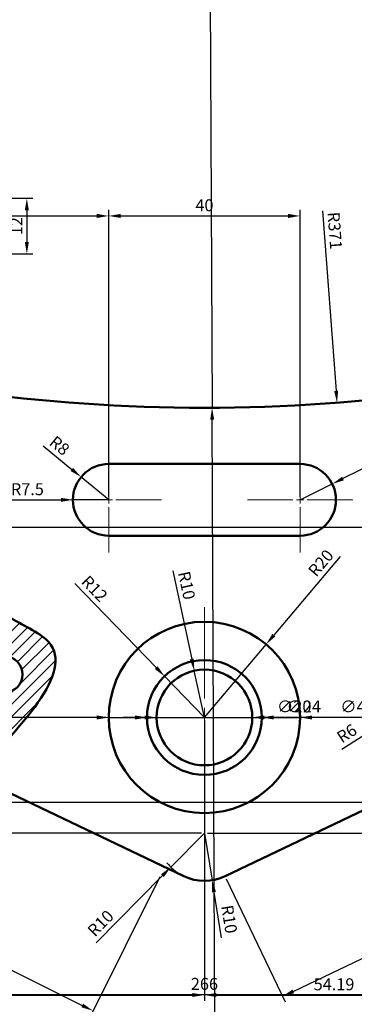
# Model space of a CAD drawing. Units: millimetres. Extents: x 1605 to 2079, y 1280 to 1879.
# Tile 4 of 7: x 1745 to 1815, y 1384 to 1589. Entities that reach past the tile are written whole.
import ezdxf

# ---------------------------------------------------------------- set-up
doc = ezdxf.new("R2010")
doc.units = ezdxf.units.MM
doc.linetypes.add('CENTER2', pattern=[28.575, 19.05, -3.175, 3.175, -3.175])
for name, color, linetype, lineweight in [('M-CNTR', 1, 'CENTER2', 18), ('M-DIMS', 2, 'Continuous', 25), ('M-HATC', 8, 'Continuous', 18), ('M-OUTL', 7, 'Continuous', 50)]:
    doc.layers.add(name, color=color, linetype=linetype, lineweight=lineweight)
doc.styles.get("Standard").update_dxf_attribs({"font": 'arial.ttf'})
doc.dimstyles.new('ISO-25', dxfattribs={"dimtxt": 2.5, "dimasz": 2.5, "dimexe": 1.25, "dimexo": 0.625, "dimtad": 1, "dimdec": 0, "dimtxsty": 'Standard', "dimcen": 2.5, "dimadec": 0, "dimazin": 0, "dimtfac": 1, "dimtdec": 0, "dimtmove": 0, "dimatfit": 3, "dimfxl": 1, "dimarcsym": 0})

# ---------------------------------------------------------------- blocks, each defined once
blk = doc.blocks.new('*U1')
at = {"layer": 'M-CNTR', "color": 0, "transparency": 16777216}
for p, q in [((0, 4), (0, 23.5)), ((-23.5, 0), (-4, 0)), ((4, 0), (23.5, 0)), ((0, -23.5), (0, -4))]:
    blk.add_line(p, q, dxfattribs=at)
at = {"layer": 'M-CNTR', "color": 0, "linetype": 'Continuous', "transparency": 16777216}
for p, q in [((-2, 0), (2, 0)), ((0, -2), (0, 2))]:
    blk.add_line(p, q, dxfattribs=at)
blk = doc.blocks.new('*U4')
at = {"layer": 'M-CNTR', "color": 0, "transparency": 16777216}
for p, q in [((0, 1.5), (0, 11)), ((-11, 0), (-1.5, 0)), ((1.5, 0), (11, 0)), ((0, -11), (0, -1.5))]:
    blk.add_line(p, q, dxfattribs=at)
at = {"layer": 'M-CNTR', "color": 0, "linetype": 'Continuous', "transparency": 16777216}
for p, q in [((-0.75, 0), (0.75, 0)), ((0, -0.75), (0, 0.75))]:
    blk.add_line(p, q, dxfattribs=at)
blk = doc.blocks.new('*U5')
at = {"layer": 'M-CNTR', "color": 0, "transparency": 16777216}
for p, q in [((0, 1.5), (0, 11)), ((-11, 0), (-1.5, 0)), ((1.5, 0), (11, 0)), ((0, -11), (0, -1.5))]:
    blk.add_line(p, q, dxfattribs=at)
at = {"layer": 'M-CNTR', "color": 0, "linetype": 'Continuous', "transparency": 16777216}
for p, q in [((-0.75, 0), (0.75, 0)), ((0, -0.75), (0, 0.75))]:
    blk.add_line(p, q, dxfattribs=at)
blk = doc.blocks.new('*D8')
at = {"layer": 'Defpoints', "color": 0, "transparency": 16777216}
for p in [(1738.95, 1552.02), (1738.95, 1540.38), (1746.29, 1540.38)]:
    blk.add_point(p, dxfattribs=at)
at = {"layer": 'M-DIMS', "color": 0, "lineweight": -2, "transparency": 16777216}
for p, q in [((1739.57, 1552.02), (1747.54, 1552.02)), ((1746.29, 1549.52), (1746.29, 1542.88)), ((1739.57, 1540.38), (1747.54, 1540.38))]:
    blk.add_line(p, q, dxfattribs=at)
at = {"layer": 'M-DIMS', "color": 0, "transparency": 16777216}
for points in [[(1745.87, 1549.52), (1746.71, 1549.52), (1746.29, 1552.02)], [(1745.87, 1542.88), (1746.71, 1542.88), (1746.29, 1540.38)]]:
    blk.add_solid(points, dxfattribs=at)
at = {"layer": 'M-DIMS', "color": 0, "transparency": 16777216, "insert": (1744.41, 1546.2), "char_height": 2.5, "attachment_point": 5, "rotation": 90}
blk.add_mtext('12', dxfattribs=at)
blk = doc.blocks.new('*D12')
at = {"layer": 'Defpoints', "color": 0, "transparency": 16777216}
for p in [(1650.42, 1488.98), (1916.42, 1488.98), (1916.42, 1385.56)]:
    blk.add_point(p, dxfattribs=at)
at = {"layer": 'M-DIMS', "color": 0, "lineweight": -2, "transparency": 16777216}
for p, q in [((1650.42, 1488.36), (1650.42, 1384.31)), ((1916.42, 1488.36), (1916.42, 1384.31)), ((1652.92, 1385.56), (1913.92, 1385.56))]:
    blk.add_line(p, q, dxfattribs=at)
at = {"layer": 'M-DIMS', "color": 0, "transparency": 16777216}
for points in [[(1652.92, 1385.97), (1652.92, 1385.14), (1650.42, 1385.56)], [(1913.92, 1385.97), (1913.92, 1385.14), (1916.42, 1385.56)]]:
    blk.add_solid(points, dxfattribs=at)
at = {"layer": 'M-DIMS', "color": 0, "transparency": 16777216, "insert": (1783.42, 1387.46), "char_height": 2.5, "attachment_point": 5}
blk.add_mtext('266', dxfattribs=at)
blk = doc.blocks.new('*D13')
at = {"layer": 'Defpoints', "color": 0, "transparency": 16777216}
for p in [(1783.42, 1419.31), (1776.39, 1412.2)]:
    blk.add_point(p, dxfattribs=at)
at = {"layer": 'M-DIMS', "color": 0, "lineweight": -2, "transparency": 16777216}
for p, q in [((1783.42, 1419.31), (1776.39, 1412.2)), ((1760.75, 1396.34), (1774.64, 1410.42))]:
    blk.add_line(p, q, dxfattribs=at)
blk.add_arc((1783.42, 1419.31), 10, 218.2245, 240.8957, dxfattribs=at)
at = {"layer": 'M-DIMS', "color": 0, "transparency": 16777216}
blk.add_solid([(1774.34, 1410.71), (1774.93, 1410.12), (1776.39, 1412.2)], dxfattribs=at)
at = {"layer": 'M-DIMS', "color": 0, "transparency": 16777216, "insert": (1761.93, 1400.24), "char_height": 2.5, "attachment_point": 5, "rotation": 45.3865}
blk.add_mtext('R10', dxfattribs=at)
blk = doc.blocks.new('*D17')
at = {"layer": 'Defpoints', "color": 0, "transparency": 16777216}
for p in [(1783.42, 1878.81), (1811.14, 1509.27)]:
    blk.add_point(p, dxfattribs=at)
at = {"layer": 'M-DIMS', "color": 0, "lineweight": -2, "transparency": 16777216}
blk.add_line((1808.13, 1549.43), (1810.96, 1511.76), dxfattribs=at)
at = {"layer": 'M-DIMS', "color": 0, "transparency": 16777216}
blk.add_solid([(1811.37, 1511.8), (1810.54, 1511.73), (1811.14, 1509.27)], dxfattribs=at)
at = {"layer": 'M-DIMS', "color": 0, "transparency": 16777216, "insert": (1810.35, 1545.24), "char_height": 2.5, "attachment_point": 5, "rotation": 274.2909}
blk.add_mtext('R371', dxfattribs=at)
blk = doc.blocks.new('*D19')
at = {"layer": 'Defpoints', "color": 0, "transparency": 16777216}
for p in [(1796.31, 1458.77), (1783.42, 1443.48)]:
    blk.add_point(p, dxfattribs=at)
at = {"layer": 'M-DIMS', "color": 0, "lineweight": -2, "transparency": 16777216}
for p, q in [((1811.78, 1477.12), (1797.92, 1460.68)), ((1783.42, 1443.48), (1796.31, 1458.77))]:
    blk.add_line(p, q, dxfattribs=at)
at = {"layer": 'M-DIMS', "color": 0, "transparency": 16777216}
blk.add_solid([(1797.6, 1460.95), (1798.24, 1460.41), (1796.31, 1458.77)], dxfattribs=at)
at = {"layer": 'M-DIMS', "color": 0, "transparency": 16777216, "insert": (1808, 1475.58), "char_height": 2.5, "attachment_point": 5, "rotation": 49.8645}
blk.add_mtext('R20', dxfattribs=at)
blk = doc.blocks.new('*D20')
at = {"layer": 'Defpoints', "color": 0, "transparency": 16777216}
for p in [(1775.07, 1452.1), (1783.42, 1443.48)]:
    blk.add_point(p, dxfattribs=at)
at = {"layer": 'M-DIMS', "color": 0, "lineweight": -2, "transparency": 16777216}
for p, q in [((1756.34, 1471.47), (1773.33, 1453.9)), ((1783.42, 1443.48), (1775.07, 1452.1))]:
    blk.add_line(p, q, dxfattribs=at)
at = {"layer": 'M-DIMS', "color": 0, "transparency": 16777216}
blk.add_solid([(1773.63, 1454.19), (1773.03, 1453.61), (1775.07, 1452.1)], dxfattribs=at)
at = {"layer": 'M-DIMS', "color": 0, "transparency": 16777216, "insert": (1760.2, 1470.19), "char_height": 2.5, "attachment_point": 5, "rotation": 314.0509}
blk.add_mtext('R12', dxfattribs=at)
blk = doc.blocks.new('*D21')
at = {"layer": 'Defpoints', "color": 0, "transparency": 16777216}
for p in [(1781.3, 1453.25), (1783.42, 1443.48)]:
    blk.add_point(p, dxfattribs=at)
at = {"layer": 'M-DIMS', "color": 0, "lineweight": -2, "transparency": 16777216}
for p, q in [((1776.78, 1474.15), (1780.77, 1455.7)), ((1783.42, 1443.48), (1781.3, 1453.25))]:
    blk.add_line(p, q, dxfattribs=at)
at = {"layer": 'M-DIMS', "color": 0, "transparency": 16777216}
blk.add_solid([(1781.18, 1455.78), (1780.36, 1455.61), (1781.3, 1453.25)], dxfattribs=at)
at = {"layer": 'M-DIMS', "color": 0, "transparency": 16777216, "insert": (1779.4, 1471.02), "char_height": 2.5, "attachment_point": 5, "rotation": 282.212}
blk.add_mtext('R10', dxfattribs=at)
blk = doc.blocks.new('*D22')
at = {"layer": 'Defpoints', "color": 0, "transparency": 16777216}
for p in [(1810.14, 1492.31), (1803.42, 1488.98)]:
    blk.add_point(p, dxfattribs=at)
at = {"layer": 'M-DIMS', "color": 0, "lineweight": -2, "transparency": 16777216}
for p, q in [((1824.04, 1499.19), (1812.38, 1493.42)), ((1803.42, 1488.98), (1810.14, 1492.31))]:
    blk.add_line(p, q, dxfattribs=at)
at = {"layer": 'M-DIMS', "color": 0, "transparency": 16777216}
blk.add_solid([(1812.19, 1493.79), (1812.56, 1493.05), (1810.14, 1492.31)], dxfattribs=at)
at = {"layer": 'M-DIMS', "color": 0, "transparency": 16777216, "insert": (1820.82, 1499.72), "char_height": 2.5, "attachment_point": 5, "rotation": 26.3503}
blk.add_mtext('R8', dxfattribs=at)
blk = doc.blocks.new('*D23')
at = {"layer": 'Defpoints', "color": 0, "transparency": 16777216}
for p in [(1757.63, 1493.75), (1763.42, 1488.98)]:
    blk.add_point(p, dxfattribs=at)
at = {"layer": 'M-DIMS', "color": 0, "lineweight": -2, "transparency": 16777216}
for p, q in [((1749.68, 1500.28), (1755.69, 1495.34)), ((1763.42, 1488.98), (1757.63, 1493.75))]:
    blk.add_line(p, q, dxfattribs=at)
at = {"layer": 'M-DIMS', "color": 0, "transparency": 16777216}
blk.add_solid([(1755.96, 1495.66), (1755.43, 1495.01), (1757.63, 1493.75)], dxfattribs=at)
at = {"layer": 'M-DIMS', "color": 0, "transparency": 16777216, "insert": (1752.93, 1500.07), "char_height": 2.5, "attachment_point": 5, "rotation": 320.5417}
blk.add_mtext('R8', dxfattribs=at)
blk = doc.blocks.new('*D24')
at = {"layer": 'Defpoints', "color": 0, "transparency": 16777216}
for p in [(1683.42, 1455.98), (1774.34, 1410.71), (1760.12, 1382.16)]:
    blk.add_point(p, dxfattribs=at)
at = {"layer": 'M-DIMS', "color": 0, "lineweight": -2, "transparency": 16777216}
for p, q in [((1683.14, 1455.42), (1668.64, 1426.31)), ((1671.44, 1426.31), (1757.89, 1383.27)), ((1774.06, 1410.15), (1759.57, 1381.04))]:
    blk.add_line(p, q, dxfattribs=at)
at = {"layer": 'M-DIMS', "color": 0, "transparency": 16777216}
for points in [[(1671.62, 1426.69), (1671.25, 1425.94), (1669.2, 1427.43)], [(1758.07, 1383.64), (1757.7, 1382.9), (1760.12, 1382.16)]]:
    blk.add_solid(points, dxfattribs=at)
at = {"layer": 'M-DIMS', "color": 0, "transparency": 16777216, "insert": (1715.51, 1406.5), "char_height": 2.5, "attachment_point": 5, "rotation": 333.531}
blk.add_mtext('102', dxfattribs=at)
blk = doc.blocks.new('*D25')
at = {"layer": 'Defpoints', "color": 0, "transparency": 16777216}
for p in [(1883.42, 1455.98), (1895.43, 1430.83), (1787.72, 1410.29)]:
    blk.add_point(p, dxfattribs=at)
at = {"layer": 'M-DIMS', "color": 0, "lineweight": -2, "transparency": 16777216}
for p, q in [((1883.69, 1455.42), (1895.96, 1429.7)), ((1801.99, 1386.22), (1893.17, 1429.75)), ((1787.99, 1409.73), (1800.27, 1384.01))]:
    blk.add_line(p, q, dxfattribs=at)
at = {"layer": 'M-DIMS', "color": 0, "transparency": 16777216}
for points in [[(1892.99, 1430.13), (1893.35, 1429.38), (1895.43, 1430.83)], [(1801.81, 1386.59), (1802.17, 1385.84), (1799.73, 1385.14)]]:
    blk.add_solid(points, dxfattribs=at)
at = {"layer": 'M-DIMS', "color": 0, "transparency": 16777216, "insert": (1846.76, 1409.7), "char_height": 2.5, "attachment_point": 5, "rotation": 25.5234}
blk.add_mtext('106', dxfattribs=at)
blk = doc.blocks.new('*D28')
at = {"layer": 'Defpoints', "color": 0, "transparency": 16777216}
for p in [(1834.3, 1451.14), (1829.05, 1447.75)]:
    blk.add_point(p, dxfattribs=at)
at = {"layer": 'M-DIMS', "color": 0, "lineweight": -2, "transparency": 16777216}
for p, q in [((1834.3, 1451.14), (1829.05, 1447.75)), ((1812.16, 1436.85), (1826.95, 1446.39))]:
    blk.add_line(p, q, dxfattribs=at)
at = {"layer": 'M-DIMS', "color": 0, "transparency": 16777216}
blk.add_solid([(1826.72, 1446.74), (1827.18, 1446.04), (1829.05, 1447.75)], dxfattribs=at)
at = {"layer": 'M-DIMS', "color": 0, "transparency": 16777216, "insert": (1813.35, 1439.88), "char_height": 2.5, "attachment_point": 5, "rotation": 32.8205}
blk.add_mtext('R6', dxfattribs=at)
blk = doc.blocks.new('*D40')
at = {"layer": 'Defpoints', "color": 0, "transparency": 16777216}
for p in [(1916.42, 1488.98), (1783.42, 1419.31), (2077.9, 1419.31)]:
    blk.add_point(p, dxfattribs=at)
at = {"layer": 'M-DIMS', "color": 0, "lineweight": -2, "transparency": 16777216}
for p, q in [((1917.04, 1488.98), (2079.15, 1488.98)), ((2077.9, 1486.48), (2077.9, 1421.81)), ((1784.04, 1419.31), (2079.15, 1419.31))]:
    blk.add_line(p, q, dxfattribs=at)
at = {"layer": 'M-DIMS', "color": 0, "transparency": 16777216}
for points in [[(2077.48, 1486.48), (2078.32, 1486.48), (2077.9, 1488.98)], [(2077.48, 1421.81), (2078.32, 1421.81), (2077.9, 1419.31)]]:
    blk.add_solid(points, dxfattribs=at)
at = {"layer": 'M-DIMS', "color": 0, "transparency": 16777216, "insert": (2076, 1454.15), "char_height": 2.5, "attachment_point": 5, "rotation": 90}
blk.add_mtext('69.67', dxfattribs=at)
blk = doc.blocks.new('*D41')
at = {"layer": 'Defpoints', "color": 0, "transparency": 16777216}
for p in [(1763.42, 1443.48), (1624.07, 1419.31), (1783.42, 1419.31)]:
    blk.add_point(p, dxfattribs=at)
at = {"layer": 'M-DIMS', "color": 0, "lineweight": -2, "transparency": 16777216}
for p, q in [((1762.79, 1443.48), (1622.82, 1443.48)), ((1624.07, 1440.98), (1624.07, 1421.81)), ((1782.79, 1419.31), (1622.82, 1419.31))]:
    blk.add_line(p, q, dxfattribs=at)
at = {"layer": 'M-DIMS', "color": 0, "transparency": 16777216}
for points in [[(1623.65, 1440.98), (1624.48, 1440.98), (1624.07, 1443.48)], [(1623.65, 1421.81), (1624.48, 1421.81), (1624.07, 1419.31)]]:
    blk.add_solid(points, dxfattribs=at)
at = {"layer": 'M-DIMS', "color": 0, "transparency": 16777216, "insert": (1622.16, 1431.4), "char_height": 2.5, "attachment_point": 5, "rotation": 90}
blk.add_mtext('24.165', dxfattribs=at)
blk = doc.blocks.new('*D42')
at = {"layer": 'Defpoints', "color": 0, "transparency": 16777216}
for p in [(1683.42, 1488.98), (1783.42, 1443.48), (1783.42, 1385.46)]:
    blk.add_point(p, dxfattribs=at)
at = {"layer": 'M-DIMS', "color": 0, "lineweight": -2, "transparency": 16777216}
for p, q in [((1683.42, 1488.36), (1683.42, 1384.21)), ((1783.42, 1442.85), (1783.42, 1384.21)), ((1685.92, 1385.46), (1780.92, 1385.46))]:
    blk.add_line(p, q, dxfattribs=at)
at = {"layer": 'M-DIMS', "color": 0, "transparency": 16777216}
for points in [[(1685.92, 1385.88), (1685.92, 1385.05), (1683.42, 1385.46)], [(1780.92, 1385.88), (1780.92, 1385.05), (1783.42, 1385.46)]]:
    blk.add_solid(points, dxfattribs=at)
at = {"layer": 'M-DIMS', "color": 0, "transparency": 16777216, "insert": (1733.42, 1387.37), "char_height": 2.5, "attachment_point": 5}
blk.add_mtext('100', dxfattribs=at)
blk = doc.blocks.new('*D43')
at = {"layer": 'Defpoints', "color": 0, "transparency": 16777216}
for p in [(1837.61, 1451.86), (1783.42, 1443.48), (1837.61, 1385.46)]:
    blk.add_point(p, dxfattribs=at)
at = {"layer": 'M-DIMS', "color": 0, "lineweight": -2, "transparency": 16777216}
for p, q in [((1837.61, 1451.24), (1837.61, 1384.21)), ((1783.42, 1442.85), (1783.42, 1384.21)), ((1785.92, 1385.46), (1835.11, 1385.46))]:
    blk.add_line(p, q, dxfattribs=at)
at = {"layer": 'M-DIMS', "color": 0, "transparency": 16777216}
for points in [[(1785.92, 1385.88), (1785.92, 1385.05), (1783.42, 1385.46)], [(1835.11, 1385.88), (1835.11, 1385.05), (1837.61, 1385.46)]]:
    blk.add_solid(points, dxfattribs=at)
at = {"layer": 'M-DIMS', "color": 0, "transparency": 16777216, "insert": (1810.51, 1387.37), "char_height": 2.5, "attachment_point": 5}
blk.add_mtext('54.19', dxfattribs=at)
blk = doc.blocks.new('*D44')
at = {"layer": 'Defpoints', "color": 0, "transparency": 16777216}
for p in [(1803.42, 1548.33), (1763.42, 1488.98), (1803.42, 1488.98)]:
    blk.add_point(p, dxfattribs=at)
at = {"layer": 'M-DIMS', "color": 0, "lineweight": -2, "transparency": 16777216}
for p, q in [((1763.42, 1489.61), (1763.42, 1549.58)), ((1765.92, 1548.33), (1800.92, 1548.33)), ((1803.42, 1489.61), (1803.42, 1549.58))]:
    blk.add_line(p, q, dxfattribs=at)
at = {"layer": 'M-DIMS', "color": 0, "transparency": 16777216}
for points in [[(1765.92, 1548.75), (1765.92, 1547.91), (1763.42, 1548.33)], [(1800.92, 1548.75), (1800.92, 1547.91), (1803.42, 1548.33)]]:
    blk.add_solid(points, dxfattribs=at)
at = {"layer": 'M-DIMS', "color": 0, "transparency": 16777216, "insert": (1783.42, 1550.23), "char_height": 2.5, "attachment_point": 5}
blk.add_mtext('40', dxfattribs=at)
blk = doc.blocks.new('*D45')
at = {"layer": 'Defpoints', "color": 0, "transparency": 16777216}
for p in [(1763.42, 1548.33), (1683.42, 1488.98), (1763.42, 1488.98)]:
    blk.add_point(p, dxfattribs=at)
at = {"layer": 'M-DIMS', "color": 0, "lineweight": -2, "transparency": 16777216}
for p, q in [((1683.42, 1489.61), (1683.42, 1549.58)), ((1685.92, 1548.33), (1760.92, 1548.33)), ((1763.42, 1489.61), (1763.42, 1549.58))]:
    blk.add_line(p, q, dxfattribs=at)
at = {"layer": 'M-DIMS', "color": 0, "transparency": 16777216}
for points in [[(1685.92, 1548.75), (1685.92, 1547.91), (1683.42, 1548.33)], [(1760.92, 1548.75), (1760.92, 1547.91), (1763.42, 1548.33)]]:
    blk.add_solid(points, dxfattribs=at)
at = {"layer": 'M-DIMS', "color": 0, "transparency": 16777216, "insert": (1723.42, 1550.23), "char_height": 2.5, "attachment_point": 5}
blk.add_mtext('80', dxfattribs=at)
blk = doc.blocks.new('*D51')
at = {"layer": 'Defpoints', "color": 0, "transparency": 16777216}
for p in [(1624.07, 1483.2), (1984.76, 1483.2), (1947.57, 1425.73)]:
    blk.add_point(p, dxfattribs=at)
at = {"layer": 'M-DIMS', "color": 0, "lineweight": -2, "transparency": 16777216}
for p, q in [((1984.13, 1483.2), (1622.82, 1483.2)), ((1624.07, 1428.23), (1624.07, 1480.7)), ((1946.94, 1425.73), (1622.82, 1425.73))]:
    blk.add_line(p, q, dxfattribs=at)
at = {"layer": 'M-DIMS', "color": 0, "transparency": 16777216}
for points in [[(1623.65, 1480.7), (1624.48, 1480.7), (1624.07, 1483.2)], [(1623.65, 1428.23), (1624.48, 1428.23), (1624.07, 1425.73)]]:
    blk.add_solid(points, dxfattribs=at)
at = {"layer": 'M-DIMS', "color": 0, "transparency": 16777216, "insert": (1622.17, 1454.47), "char_height": 2.5, "attachment_point": 5, "rotation": 90}
blk.add_mtext('57.47', dxfattribs=at)
blk = doc.blocks.new('*D64')
at = {"layer": 'Defpoints', "color": 0, "transparency": 16777216}
for p in [(1763.42, 1443.48), (1803.42, 1443.48)]:
    blk.add_point(p, dxfattribs=at)
at = {"layer": 'M-DIMS', "color": 0, "lineweight": -2, "transparency": 16777216}
for p, q in [((1760.92, 1443.48), (1758.42, 1443.48)), ((1763.42, 1443.48), (1803.42, 1443.48)), ((1819.19, 1443.48), (1805.92, 1443.48))]:
    blk.add_line(p, q, dxfattribs=at)
at = {"layer": 'M-DIMS', "color": 0, "transparency": 16777216}
for points in [[(1760.92, 1443.9), (1760.92, 1443.06), (1763.42, 1443.48)], [(1805.92, 1443.9), (1805.92, 1443.06), (1803.42, 1443.48)]]:
    blk.add_solid(points, dxfattribs=at)
at = {"layer": 'M-DIMS', "color": 0, "transparency": 16777216, "insert": (1815.42, 1445.45), "char_height": 2.5, "attachment_point": 5, "rotation": 359.9999}
blk.add_mtext('∅40', dxfattribs=at)
blk = doc.blocks.new('*D65')
at = {"layer": 'Defpoints', "color": 0, "transparency": 16777216}
for p in [(1771.42, 1443.48), (1795.42, 1443.48)]:
    blk.add_point(p, dxfattribs=at)
at = {"layer": 'M-DIMS', "color": 0, "lineweight": -2, "transparency": 16777216}
for p, q in [((1768.92, 1443.48), (1766.42, 1443.48)), ((1771.42, 1443.48), (1795.42, 1443.48)), ((1807.96, 1443.48), (1797.92, 1443.48))]:
    blk.add_line(p, q, dxfattribs=at)
at = {"layer": 'M-DIMS', "color": 0, "transparency": 16777216}
for points in [[(1768.92, 1443.9), (1768.92, 1443.06), (1771.42, 1443.48)], [(1797.92, 1443.9), (1797.92, 1443.06), (1795.42, 1443.48)]]:
    blk.add_solid(points, dxfattribs=at)
at = {"layer": 'M-DIMS', "color": 0, "transparency": 16777216, "insert": (1804.19, 1445.45), "char_height": 2.5, "attachment_point": 5, "rotation": 359.9999}
blk.add_mtext('∅24', dxfattribs=at)
blk = doc.blocks.new('*D66')
at = {"layer": 'Defpoints', "color": 0, "transparency": 16777216}
for p in [(1773.42, 1443.48), (1793.42, 1443.48)]:
    blk.add_point(p, dxfattribs=at)
at = {"layer": 'M-DIMS', "color": 0, "lineweight": -2, "transparency": 16777216}
for p, q in [((1770.92, 1443.48), (1768.42, 1443.48)), ((1773.42, 1443.48), (1793.42, 1443.48)), ((1805.96, 1443.48), (1795.92, 1443.48))]:
    blk.add_line(p, q, dxfattribs=at)
at = {"layer": 'M-DIMS', "color": 0, "transparency": 16777216}
for points in [[(1770.92, 1443.9), (1770.92, 1443.06), (1773.42, 1443.48)], [(1795.92, 1443.9), (1795.92, 1443.06), (1793.42, 1443.48)]]:
    blk.add_solid(points, dxfattribs=at)
at = {"layer": 'M-DIMS', "color": 0, "transparency": 16777216, "insert": (1802.19, 1445.45), "char_height": 2.5, "attachment_point": 5, "rotation": 359.9999}
blk.add_mtext('∅20', dxfattribs=at)
blk = doc.blocks.new('*D68')
at = {"layer": 'Defpoints', "color": 0, "transparency": 16777216}
for p in [(1755.92, 1488.98), (1763.42, 1488.98)]:
    blk.add_point(p, dxfattribs=at)
at = {"layer": 'M-DIMS', "color": 0, "lineweight": -2, "transparency": 16777216}
for p, q in [((1737.29, 1488.98), (1753.42, 1488.98)), ((1763.42, 1488.98), (1755.92, 1488.98))]:
    blk.add_line(p, q, dxfattribs=at)
at = {"layer": 'M-DIMS', "color": 0, "transparency": 16777216}
blk.add_solid([(1753.42, 1489.4), (1753.42, 1488.56), (1755.92, 1488.98)], dxfattribs=at)
at = {"layer": 'M-DIMS', "color": 0, "transparency": 16777216, "insert": (1744.1, 1490.88), "char_height": 2.5, "attachment_point": 5, "rotation": 359.997}
blk.add_mtext('2X R7.5', dxfattribs=at)
blk = doc.blocks.new('*D71')
at = {"layer": 'Defpoints', "color": 0, "transparency": 16777216}
for p in [(1783.42, 1878.81), (1785.02, 1508.24)]:
    blk.add_point(p, dxfattribs=at)
at = {"layer": 'M-DIMS', "color": 0, "lineweight": -2, "transparency": 16777216}
for p, q in [((1783.42, 1878.81), (1785.02, 1508.24)), ((1786.01, 1279.86), (1785.03, 1505.74))]:
    blk.add_line(p, q, dxfattribs=at)
at = {"layer": 'M-DIMS', "color": 0, "transparency": 16777216}
blk.add_solid([(1785.45, 1505.74), (1784.61, 1505.73), (1785.02, 1508.24)], dxfattribs=at)
at = {"layer": 'M-DIMS', "color": 0, "transparency": 16777216, "insert": (1787.88, 1285.9), "char_height": 2.5, "attachment_point": 5, "rotation": 270.2478}
blk.add_mtext('R370.6', dxfattribs=at)
blk = doc.blocks.new('*D72')
at = {"layer": 'Defpoints', "color": 0, "transparency": 16777216}
for p in [(1783.42, 1419.31), (1785.03, 1409.44)]:
    blk.add_point(p, dxfattribs=at)
at = {"layer": 'M-DIMS', "color": 0, "lineweight": -2, "transparency": 16777216}
for p, q in [((1783.42, 1419.31), (1785.03, 1409.44)), ((1786.99, 1397.39), (1785.43, 1406.98))]:
    blk.add_line(p, q, dxfattribs=at)
at = {"layer": 'M-DIMS', "color": 0, "transparency": 16777216}
blk.add_solid([(1785.84, 1407.04), (1785.02, 1406.91), (1785.03, 1409.44)], dxfattribs=at)
at = {"layer": 'M-DIMS', "color": 0, "transparency": 16777216, "insert": (1788.29, 1401.26), "char_height": 2.5, "attachment_point": 5, "rotation": 279.2618}
blk.add_mtext('R10', dxfattribs=at)

msp = doc.modelspace()

# ---------------------------------------------------------------- hatches: boundary and pattern name
at = {"layer": 'M-HATC'}
h = msp.add_hatch(dxfattribs=at)
h.set_pattern_fill('ANSI31', color=256, scale=0.57)
edge = h.paths.add_edge_path()
edge.add_spline(control_points=[(1735.0746, 1431.3148), (1745.9833, 1442.5727), (1760.2498, 1457.2961), (1736.484, 1465.9494), (1733.1843, 1487.5731), (1732.3186, 1503.2284), (1731.8425, 1511.8393)], knot_values=[0, 0, 0, 0, 32.31065912, 42.25647348, 64.01517543, 90.61240603, 90.61240603, 90.61240603, 90.61240603], degree=3, periodic=0)
edge.add_arc((1783.4159, 1878.8069), 370.5739, 256.032866, 262.000081, ccw=False)
edge.add_arc((1683.4159, 1488.9806), 32, 0, 70.738174, ccw=False)
edge.add_arc((1683.4159, 1488.9806), 32, -90, 0, ccw=False)
edge.add_line((1683.4159, 1456.9806), (1683.4159, 1455.9806))
edge.add_line((1683.4159, 1455.9806), (1735.0746, 1431.3148))
h.paths.add_polyline_path([(1726.6663, 1456.2378), (1741.6663, 1456.2378, -1), (1741.6663, 1448.7378), (1726.6663, 1448.7378, -1)], flags=16)
h.paths.add_polyline_path([(1731.4787, 1442.133), (1736.6134, 1442.133), (1736.6134, 1447.2848), (1731.4787, 1447.2848)], flags=24)
h.paths.add_polyline_path([(1713.1734, 1457.2688), (1718.4539, 1455.0843), (1720.4233, 1459.8448), (1715.1428, 1462.0293)], flags=24)

# ---------------------------------------------------------------- linework, layer by layer
at = {"layer": 'M-OUTL'}
for p, q in [((1783.4159, 1496.4806), (1763.4159, 1496.4806)), ((1803.4159, 1496.4806), (1783.4159, 1496.4806)), ((1763.4159, 1481.4806), (1803.4159, 1481.4806)), ((1683.4159, 1455.9806), (1779.1071, 1410.2904)), ((1787.7246, 1410.2904), (1883.4159, 1455.9806))]:
    msp.add_line(p, q, dxfattribs=at)
for radius in [20, 12, 10]:
    msp.add_circle((1783.4159, 1443.479), radius, dxfattribs=at)
for centre, radius, start, end in [((1783.4159, 1878.8069), 370.5739, 254.344556, 285.655444), ((1763.4159, 1488.9806), 7.5, 90, 270), ((1803.4159, 1488.9806), 7.5, 270, 90), ((1741.6663, 1452.4878), 3.75, 270, 90), ((1783.4159, 1419.3145), 10, 244.476648, 295.523352)]:
    msp.add_arc(centre, radius, start, end, dxfattribs=at)
msp.add_open_spline([(1731.8425, 1511.8393), (1732.3186, 1503.2284), (1733.1843, 1487.5731), (1736.484, 1465.9494), (1760.2498, 1457.2961), (1745.9833, 1442.5727), (1735.0746, 1431.3148)], degree=3, knots=[0, 0, 0, 0, 26.5972306, 48.35593255, 58.30174691, 90.61240603, 90.61240603, 90.61240603, 90.61240603], dxfattribs=at)

# ---------------------------------------------------------------- block references
at = {"layer": 'M-CNTR'}
for name, p in [('*U5', (1763.4159, 1488.9806)), ('*U4', (1803.4159, 1488.9806)), ('*U1', (1783.4159, 1443.479))]:
    msp.add_blockref(name, p, dxfattribs=at)

# ---------------------------------------------------------------- dimensions: what is measured, and where the dimension line sits
at = {"layer": 'M-DIMS'}
for center, mpoint, override, picture, middle in [((1783.4159, 1878.8069), (1811.1421, 1509.2717), {"dimclrd": 0, "dimclre": 0, "dimclrt": 0}, '*D17', (1808.4541, 1545.0966)), ((1783.4159, 1878.8069), (1785.0189, 1508.2365), {"dimdec": 1, "dimlfac": 1, "dimrnd": 0, "dimzin": 0, "dimdsep": 46, "dimlunit": 2}, '*D71', (1785.9807, 1285.8942)), ((1803.4159, 1488.9806), (1810.1366, 1492.3095), {"dimclrd": 0, "dimclre": 0, "dimclrt": 0}, '*D22', (1821.6668, 1498.0207)), ((1783.4159, 1443.479), (1796.3078, 1458.7695), {"dimclrd": 0, "dimclre": 0, "dimclrt": 0}, '*D19', (1809.4513, 1474.3583)), ((1783.4159, 1443.479), (1781.3006, 1453.2527), {"dimclrd": 0, "dimclre": 0, "dimclrt": 0}, '*D21', (1777.5414, 1470.6221)), ((1783.4159, 1443.479), (1775.0723, 1452.1037), {"dimclrd": 0, "dimclre": 0, "dimclrt": 0}, '*D20', (1758.8442, 1468.8785)), ((1834.3044, 1451.1354), (1829.0511, 1447.7473), {"dimclrd": 0, "dimclre": 0, "dimclrt": 0}, '*D28', (1814.3783, 1438.2839)), ((1783.4159, 1419.3145), (1776.3926, 1412.1958), {"dimclrd": 0, "dimclre": 0, "dimclrt": 0}, '*D13', (1763.2795, 1398.9046))]:
    dim = msp.add_radius_dim(center=center, mpoint=mpoint, dimstyle='ISO-25', override=override, dxfattribs=at)
    dim.commit()
    dim.dimension.update_dxf_attribs({"geometry": picture, "text_midpoint": middle, "dimtype": 164})
for base, p1, p2, override, picture, middle in [((1763.4159, 1548.3306), (1683.4159, 1488.9806), (1763.4159, 1488.9806), {"dimdec": 0, "dimlfac": 1, "dimrnd": 0, "dimzin": 0, "dimdsep": 46, "dimlunit": 2}, '*D45', (1723.4159, 1550.232)), ((1803.4159, 1548.3306), (1763.4159, 1488.9806), (1803.4159, 1488.9806), {"dimdec": 0, "dimlfac": 1, "dimrnd": 0, "dimzin": 0, "dimdsep": 46, "dimlunit": 2}, '*D44', (1783.4159, 1550.232)), ((1916.4159, 1385.5558), (1650.4159, 1488.9806), (1916.4159, 1488.9806), {"dimclrd": 0, "dimclre": 0, "dimclrt": 0}, '*D12', (1783.4159, 1387.4572)), ((1783.4159, 1385.4644), (1683.4159, 1488.9806), (1783.4159, 1443.479), {"dimdec": 0, "dimlfac": 1, "dimrnd": 0, "dimzin": 0, "dimdsep": 46, "dimlunit": 2}, '*D42', (1733.4159, 1387.3659)), ((1837.6066, 1385.4644), (1783.4159, 1443.479), (1837.6066, 1451.8622), {"dimdec": 2, "dimlfac": 1, "dimrnd": 0, "dimzin": 0, "dimdsep": 46, "dimlunit": 2}, '*D43', (1810.5112, 1387.3659))]:
    dim = msp.add_linear_dim(base=base, p1=p1, p2=p2, dimstyle='ISO-25', override=override, dxfattribs=at)
    dim.commit()
    dim.dimension.update_dxf_attribs({"geometry": picture, "text_midpoint": middle})
for base, p1, p2, override, picture, middle in [((1746.2909, 1540.3843), (1738.9458, 1552.0206), (1738.9458, 1540.3843), {"dimclrd": 0, "dimclre": 0, "dimclrt": 0}, '*D8', (1744.4108, 1546.2025)), ((2077.8984, 1419.3145), (1916.4159, 1488.9806), (1783.4159, 1419.3145), {"dimdec": 2, "dimlfac": 1, "dimrnd": 0, "dimzin": 0, "dimdsep": 46, "dimlunit": 2}, '*D40', (2075.997, 1454.1475)), ((1624.0659, 1483.2046), (1947.5688, 1425.7344), (1984.7564, 1483.2046), {"dimdec": 2, "dimlfac": 1, "dimrnd": 0, "dimzin": 0, "dimdsep": 46, "dimlunit": 2}, '*D51', (1622.1695, 1454.4695)), ((1624.06586, 1419.31445), (1763.41586, 1443.47902), (1783.41586, 1419.31445), {"dimdec": 3, "dimlfac": 1, "dimrnd": 0, "dimzin": 0, "dimdsep": 46, "dimlunit": 2}, '*D41', (1622.16442, 1431.39674))]:
    dim = msp.add_linear_dim(base=base, p1=p1, p2=p2, angle=90, dimstyle='ISO-25', override=override, dxfattribs=at)
    dim.commit()
    dim.dimension.update_dxf_attribs({"geometry": picture, "text_midpoint": middle})
for center, mpoint, override, picture, middle in [((1763.4159, 1488.9806), (1757.6252, 1493.747), {"dimclrd": 0, "dimclre": 0, "dimclrt": 0}, '*D23', (1752.9323, 1500.0725)), ((1783.4159, 1419.3145), (1785.0253, 1409.4448), {"dimdec": 0, "dimlfac": 1, "dimrnd": 0, "dimzin": 0, "dimdsep": 46, "dimlunit": 2}, '*D72', (1788.2873, 1401.2555))]:
    dim = msp.add_radius_dim(center=center, mpoint=mpoint, dimstyle='ISO-25', override=override, dxfattribs=at)
    dim.commit()
    dim.dimension.update_dxf_attribs({"geometry": picture, "text_midpoint": middle})
dim = msp.add_radius_dim(center=(1763.4159, 1488.9806), mpoint=(1755.9159, 1488.981), text='2X <>', dimstyle='ISO-25', override={"dimdec": 1, "dimlfac": 1, "dimrnd": 0, "dimzin": 0, "dimdsep": 46, "dimlunit": 2}, dxfattribs=at)
dim.commit()
dim.dimension.update_dxf_attribs({"geometry": '*D68', "text_midpoint": (1744.1023, 1490.8831)})
for p1, p2, distance, picture, middle in [((1683.4159, 1455.9806), (1774.3402, 1410.7088), -31.8951, '*D24', (1715.5095, 1406.4951)), ((1787.7246, 1410.2904), (1883.4159, 1455.9806), -27.8723, '*D25', (1846.7605, 1409.6992))]:
    dim = msp.add_aligned_dim(p1=p1, p2=p2, distance=distance, dimstyle='ISO-25', override={"dimclrd": 0, "dimclre": 0, "dimclrt": 0}, dxfattribs=at)
    dim.commit()
    dim.dimension.update_dxf_attribs({"geometry": picture, "text_midpoint": middle})
dim = msp.add_diameter_dim_2p(p1=(1763.4159, 1443.479), p2=(1803.4159, 1443.479), dimstyle='ISO-25', override={"dimdec": 0, "dimlfac": 1, "dimrnd": 0, "dimzin": 0, "dimdsep": 46, "dimlunit": 2}, dxfattribs=at)
dim.commit()
dim.dimension.update_dxf_attribs({"geometry": '*D64', "text_midpoint": (1815.4159, 1443.479), "dimtype": 163})
for p1, p2, picture, middle in [((1771.4159, 1443.479), (1795.4159, 1443.479), '*D65', (1804.1863, 1443.479)), ((1773.4159, 1443.479), (1793.4159, 1443.479), '*D66', (1802.1872, 1443.479))]:
    dim = msp.add_diameter_dim_2p(p1=p1, p2=p2, dimstyle='ISO-25', override={"dimdec": 0, "dimlfac": 1, "dimrnd": 0, "dimzin": 0, "dimdsep": 46, "dimlunit": 2}, dxfattribs=at)
    dim.commit()
    dim.dimension.update_dxf_attribs({"geometry": picture, "text_midpoint": middle})

doc.saveas('drawing.dxf')
